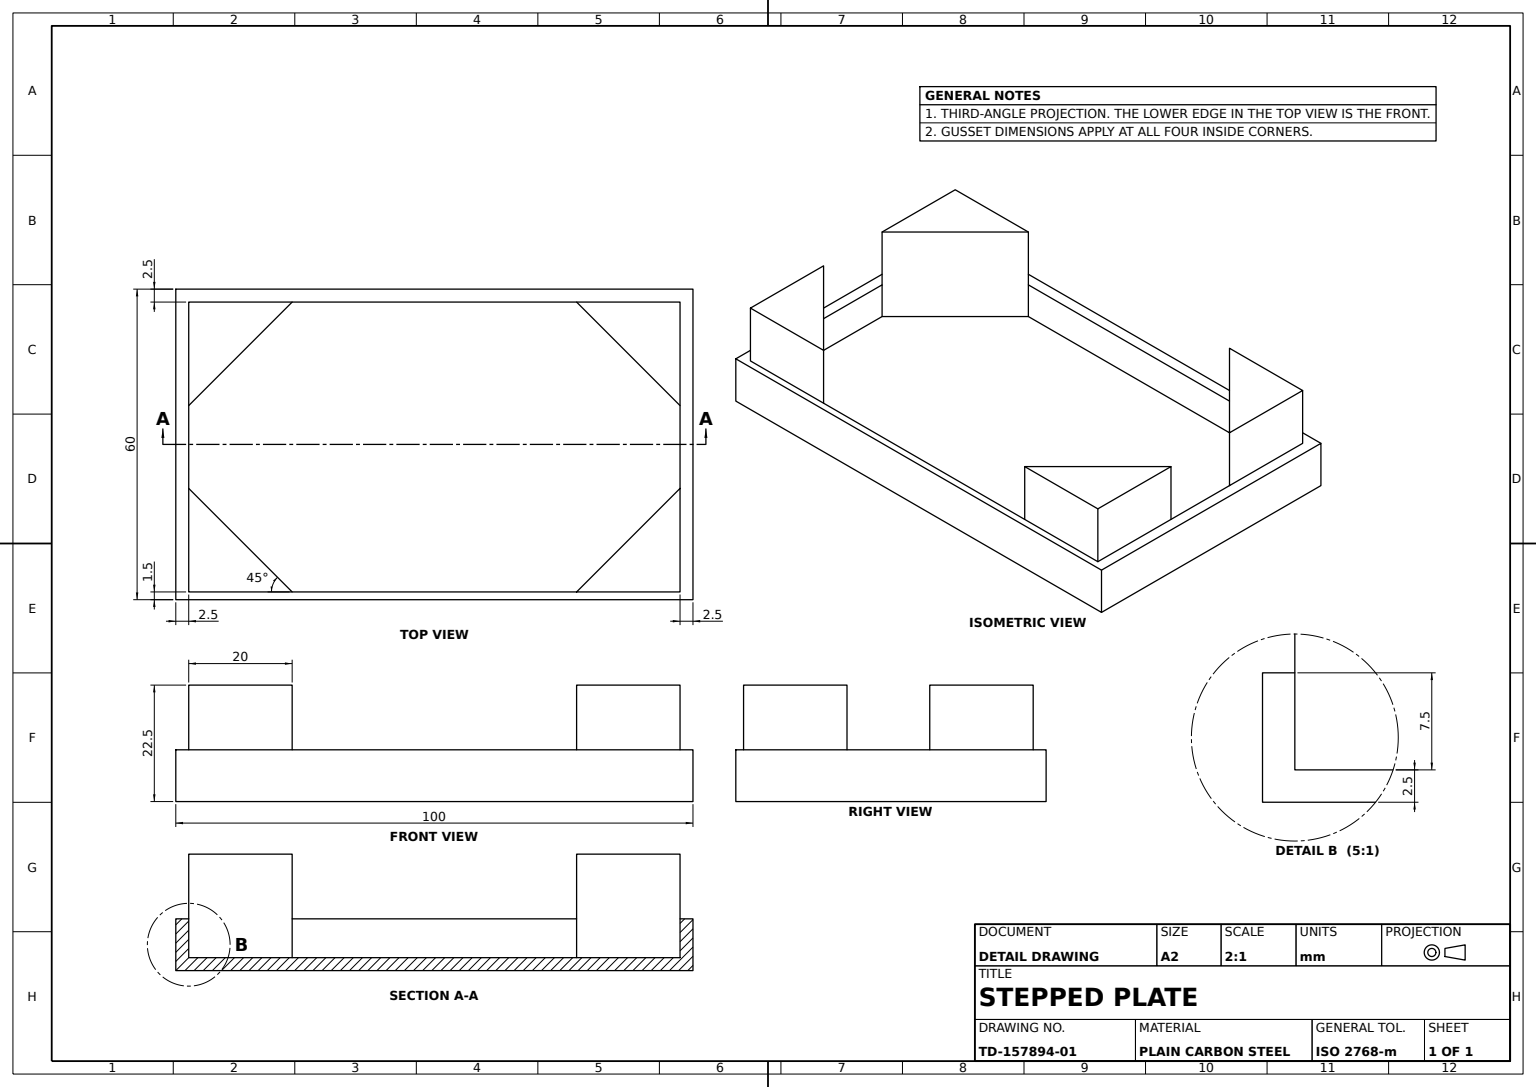
from build123d import *

# Parameters (mm, degrees)
BASE_PLATE_PROFILE_W      = 100
BASE_PLATE_PROFILE_H      = 60
BASE_PLATE_2_5MM_DEPTH    = 2.5
RIM_WALL_PROFILE_W        = 100
RIM_WALL_PROFILE_H        = 60
RIM_WALL_PROFILE_W_2      = 95
RIM_WALL_PROFILE_H_2      = 56
RIM_WALL_7_5MM_DEPTH      = 7.5
CORNER_GUSSETS_20MM_DEPTH = 20


with BuildPart() as part:
    # Base Plate Profile → Base Plate 2.5mm (new body)
    with BuildSketch(Plane.XY):
        with Locations((50, 30)):
            Rectangle(BASE_PLATE_PROFILE_W, BASE_PLATE_PROFILE_H)
    extrude(amount=BASE_PLATE_2_5MM_DEPTH)

    # Rim Wall Profile → Rim Wall 7.5mm (add)
    with BuildSketch(Plane.XY.offset(2.5)):
        with Locations((50, 30)):
            Rectangle(RIM_WALL_PROFILE_W, RIM_WALL_PROFILE_H)
        with Locations((50, 29.5)):
            Rectangle(RIM_WALL_PROFILE_W_2, RIM_WALL_PROFILE_H_2, mode=Mode.SUBTRACT)
    extrude(amount=RIM_WALL_7_5MM_DEPTH)

    # Corner Gusset Profile → Corner Gussets 20mm (add)
    with BuildSketch(Plane.XY.offset(2.5)):
        Polygon((2.5, 57.5), (22.5, 57.5), (2.5, 37.5), align=None)
        Polygon((2.5, 1.5), (22.5, 1.5), (2.5, 21.5), align=None)
        Polygon((97.5, 57.5), (77.5, 57.5), (97.5, 37.5), align=None)
        Polygon((97.5, 1.5), (77.5, 1.5), (97.5, 21.5), align=None)
    extrude(amount=CORNER_GUSSETS_20MM_DEPTH)


solid = part.part
